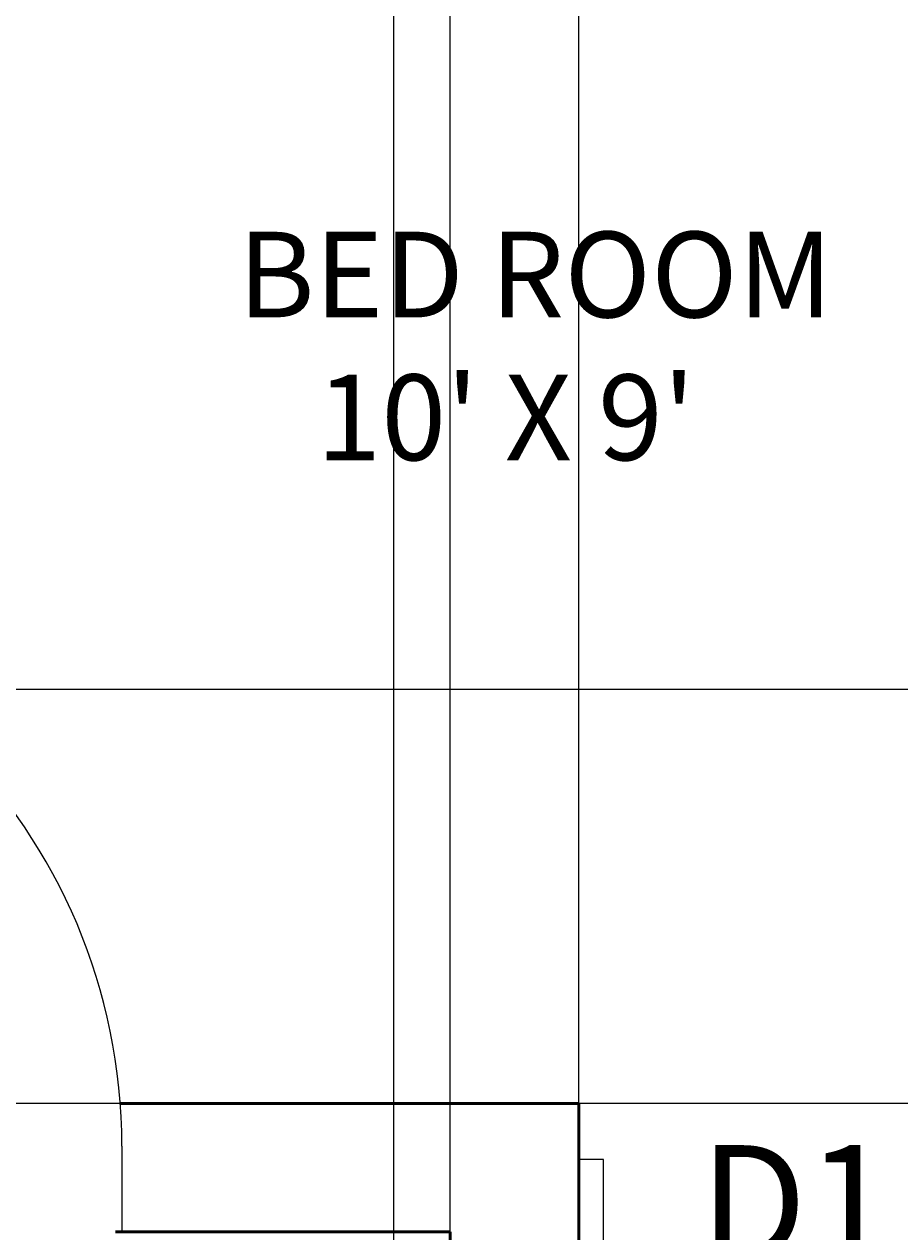
# Model space of a CAD drawing. Units: inches. Extents: x 37 to 824, y -700 to 234.
# Tile 70 of 77: x 332 to 394, y 75 to 160. Entities that reach past the tile are written whole.
import ezdxf

# ---------------------------------------------------------------- set-up
doc = ezdxf.new("R2010")
doc.units = ezdxf.units.IN
doc.header["$MEASUREMENT"] = 0
for name, color, linetype, lineweight in [('A-ANNO-DIMS', 2, 'Continuous', 18), ('A-ANNO-TEXT', 7, 'Continuous', 18), ('A-AREA-IDEN', 3, 'Continuous', 18), ('A-DOOR', 4, 'Continuous', 25), ('A-WALL', 2, 'Continuous', 50)]:
    doc.layers.add(name, color=color, linetype=linetype, lineweight=lineweight)
doc.styles.get("Standard").update_dxf_attribs({"font": 'arial.ttf'})
doc.dimstyles.get("Standard").update_dxf_attribs({"dimtxt": 0.18, "dimasz": 0.18, "dimexe": 0.18, "dimexo": 0.0625, "dimgap": 0.09, "dimtad": 0, "dimtih": 1, "dimtoh": 1, "dimdec": 1, "dimzin": 0, "dimdsep": 46, "dimlunit": 4, "dimtxsty": 'Standard', "dimcen": 0.09, "dimadec": 0, "dimazin": 0, "dimtfac": 1, "dimtdec": 1, "dimtofl": 0, "dimtmove": 0, "dimatfit": 3, "dimfxl": 1, "dimtolj": 1, "dimtzin": 0, "dimarcsym": 0})

# ---------------------------------------------------------------- blocks, each defined once
blk = doc.blocks.new('*U6')
for p, q in [((-750, 0), (-750, -100)), ((0, 0), (0, -100))]:
    blk.add_line(p, q)
blk.add_lwpolyline([(0, 0), (0, 750), (-43.75, 750), (-43.75, 0)], close=True)
blk.add_arc((0, 0), 750, 90, 180)
blk = doc.blocks.new('*U2')
for p, q in [((-40, 0), (-40, 6)), ((0, 0), (0, 6))]:
    blk.add_line(p, q)
blk.add_lwpolyline([(0, 0), (0, -40), (-1.75, -40), (-1.75, 0)], close=True)
blk.add_arc((0, 0), 40, 180, 270)
blk = doc.blocks.new('*D60')
at = {"layer": 'A-ANNO-DIMS', "color": 0, "lineweight": -2, "ltscale": 0.5, "transparency": 16777216}
for p, q in [((419.015, 113.09), (78.159, 113.09)), ((78.339, 112.91), (78.339, 98.772)), ((78.339, 84.27), (78.339, 98.409)), ((419.015, 84.09), (78.159, 84.09))]:
    blk.add_line(p, q, dxfattribs=at)
at = {"layer": 'A-ANNO-DIMS', "color": 0, "ltscale": 0.5, "transparency": 16777216}
for points in [[(78.309, 112.91), (78.369, 112.91), (78.339, 113.09)], [(78.309, 84.27), (78.369, 84.27), (78.339, 84.09)]]:
    blk.add_solid(points, dxfattribs=at)
at = {"layer": 'Defpoints', "color": 0, "ltscale": 0.5, "transparency": 16777216}
for p in [(78.339, 113.09), (419.077, 113.09), (419.077, 84.09)]:
    blk.add_point(p, dxfattribs=at)
at = {"layer": 'A-ANNO-DIMS', "color": 0, "ltscale": 0.5, "transparency": 16777216, "insert": (78.339, 98.59), "char_height": 0.18, "attachment_point": 5}
blk.add_mtext('\\A1;2\'-5"', dxfattribs=at)
blk = doc.blocks.new('*D74')
at = {"layer": 'A-ANNO-DIMS', "color": 0, "lineweight": -2, "ltscale": 0.5, "transparency": 16777216}
for p, q in [((371.077, 84.153), (371.077, 234.17)), ((371.257, 233.99), (385.3, 233.99)), ((400.425, 233.99), (386.381, 233.99)), ((400.605, 84.153), (400.605, 234.17))]:
    blk.add_line(p, q, dxfattribs=at)
at = {"layer": 'A-ANNO-DIMS', "color": 0, "ltscale": 0.5, "transparency": 16777216}
for points in [[(371.257, 234.02), (371.257, 233.96), (371.077, 233.99)], [(400.425, 234.02), (400.425, 233.96), (400.605, 233.99)]]:
    blk.add_solid(points, dxfattribs=at)
at = {"layer": 'Defpoints', "color": 0, "ltscale": 0.5, "transparency": 16777216}
for p in [(400.605, 233.99), (371.077, 84.09), (400.605, 84.09)]:
    blk.add_point(p, dxfattribs=at)
at = {"layer": 'A-ANNO-DIMS', "color": 0, "ltscale": 0.5, "transparency": 16777216, "insert": (385.841, 233.99), "char_height": 0.18, "attachment_point": 5}
blk.add_mtext('\\A1;2\'-5 1/2"', dxfattribs=at)
blk = doc.blocks.new('*D78')
at = {"layer": 'A-ANNO-DIMS', "color": 0, "lineweight": -2, "ltscale": 0.5, "transparency": 16777216}
for p, q in [((290.077, 15.153), (290.077, 234.17)), ((290.257, 233.99), (325.747, 233.99)), ((361.897, 233.99), (326.407, 233.99)), ((362.077, 15.153), (362.077, 234.17))]:
    blk.add_line(p, q, dxfattribs=at)
at = {"layer": 'A-ANNO-DIMS', "color": 0, "ltscale": 0.5, "transparency": 16777216}
for points in [[(290.257, 234.02), (290.257, 233.96), (290.077, 233.99)], [(361.897, 234.02), (361.897, 233.96), (362.077, 233.99)]]:
    blk.add_solid(points, dxfattribs=at)
at = {"layer": 'Defpoints', "color": 0, "ltscale": 0.5, "transparency": 16777216}
for p in [(362.077, 233.99), (290.077, 15.09), (362.077, 15.09)]:
    blk.add_point(p, dxfattribs=at)
at = {"layer": 'A-ANNO-DIMS', "color": 0, "ltscale": 0.5, "transparency": 16777216, "insert": (326.077, 233.99), "char_height": 0.18, "attachment_point": 5}
blk.add_mtext('\\A1;6\'-0"', dxfattribs=at)
blk = doc.blocks.new('*D82')
at = {"layer": 'A-ANNO-DIMS', "color": 0, "lineweight": -2, "ltscale": 0.5, "transparency": 16777216}
for p, q in [((299.077, -206.847), (299.077, 234.17)), ((299.257, 233.99), (328.202, 233.99)), ((357.952, 233.99), (329.008, 233.99)), ((358.132, -206.847), (358.132, 234.17))]:
    blk.add_line(p, q, dxfattribs=at)
at = {"layer": 'A-ANNO-DIMS', "color": 0, "ltscale": 0.5, "transparency": 16777216}
for points in [[(299.257, 234.02), (299.257, 233.96), (299.077, 233.99)], [(357.952, 234.02), (357.952, 233.96), (358.132, 233.99)]]:
    blk.add_solid(points, dxfattribs=at)
at = {"layer": 'Defpoints', "color": 0, "ltscale": 0.5, "transparency": 16777216}
for p in [(358.132, 233.99), (299.077, -206.91), (358.132, -206.91)]:
    blk.add_point(p, dxfattribs=at)
at = {"layer": 'A-ANNO-DIMS', "color": 0, "ltscale": 0.5, "transparency": 16777216, "insert": (328.605, 233.99), "char_height": 0.18, "attachment_point": 5}
blk.add_mtext('\\A1;4\'-11"', dxfattribs=at)
blk = doc.blocks.new('*D83')
at = {"layer": 'A-ANNO-DIMS', "color": 0, "lineweight": -2, "ltscale": 0.5, "transparency": 16777216}
for p, q in [((358.132, -206.847), (358.132, 234.17)), ((358.312, 233.99), (388.275, 233.99)), ((418.897, 233.99), (388.934, 233.99)), ((419.077, -206.847), (419.077, 234.17))]:
    blk.add_line(p, q, dxfattribs=at)
at = {"layer": 'A-ANNO-DIMS', "color": 0, "ltscale": 0.5, "transparency": 16777216}
for points in [[(358.312, 234.02), (358.312, 233.96), (358.132, 233.99)], [(418.897, 234.02), (418.897, 233.96), (419.077, 233.99)]]:
    blk.add_solid(points, dxfattribs=at)
at = {"layer": 'Defpoints', "color": 0, "ltscale": 0.5, "transparency": 16777216}
for p in [(419.077, 233.99), (358.132, -206.91), (419.077, -206.91)]:
    blk.add_point(p, dxfattribs=at)
at = {"layer": 'A-ANNO-DIMS', "color": 0, "ltscale": 0.5, "transparency": 16777216, "insert": (388.605, 233.99), "char_height": 0.18, "attachment_point": 5}
blk.add_mtext('\\A1;5\'-1"', dxfattribs=at)

msp = doc.modelspace()

# ---------------------------------------------------------------- linework, layer by layer
at = {"layer": 'A-WALL'}
for p, q in [((371.077, 84.09), (338.964, 84.09)), ((371.077, 15.09), (371.077, 84.09)), ((362.077, 75.09), (338.625, 75.09)), ((362.077, 15.09), (362.077, 75.09))]:
    msp.add_line(p, q, dxfattribs=at)

# ---------------------------------------------------------------- block references
at = {"layer": 'A-DOOR', "rotation": 180}
msp.add_blockref('*U2', (299.077, 81.09), dxfattribs=at)
at = {"layer": 'A-DOOR', "xscale": 0.0393700787401575, "yscale": 0.0393700787401575, "zscale": 0.0393700787401575, "rotation": 180}
msp.add_blockref('*U6', (371.077, 80.153), dxfattribs=at)

# ---------------------------------------------------------------- texts
at = {"layer": 'A-ANNO-TEXT'}
msp.add_text('D1', height=8, dxfattribs=at).set_placement((379.536, 73.162))
at = {"layer": 'A-AREA-IDEN', "insert": (347.2, 145.143), "char_height": 6, "attachment_point": 1}
msp.add_mtext_dynamic_manual_height_columns("BED ROOM\\P   10' X 9'", width=88.32168, gutter_width=1, heights=[0], dxfattribs=at)

# ---------------------------------------------------------------- dimensions: what is measured, and where the dimension line sits
at = {"layer": 'A-ANNO-DIMS', "ltscale": 0.5}
for base, p1, p2, picture, middle in [((362.077, 233.99), (290.077, 15.09), (362.077, 15.09), '*D78', (326.077, 233.99)), ((358.132, 233.99), (299.077, -206.91), (358.132, -206.91), '*D82', (328.605, 233.99)), ((419.077, 233.99), (358.132, -206.91), (419.077, -206.91), '*D83', (388.605, 233.99)), ((400.605, 233.99), (371.077, 84.09), (400.605, 84.09), '*D74', (385.841, 233.99))]:
    dim = msp.add_linear_dim(base=base, p1=p1, p2=p2, dimstyle='Standard', override={"dimdec": 1, "dimlfac": 1, "dimrnd": 0, "dimzin": 1, "dimdsep": 46, "dimlunit": 4, "dimfrac": 2}, dxfattribs=at)
    dim.commit()
    dim.dimension.update_dxf_attribs({"geometry": picture, "text_midpoint": middle})
dim = msp.add_linear_dim(base=(78.339, 113.09), p1=(419.077, 84.09), p2=(419.077, 113.09), angle=90, dimstyle='Standard', override={"dimdec": 1, "dimlfac": 1, "dimrnd": 0, "dimzin": 1, "dimdsep": 46, "dimlunit": 4, "dimfrac": 2}, dxfattribs=at)
dim.commit()
dim.dimension.update_dxf_attribs({"geometry": '*D60', "text_midpoint": (78.339, 98.59)})

doc.saveas('drawing.dxf')
